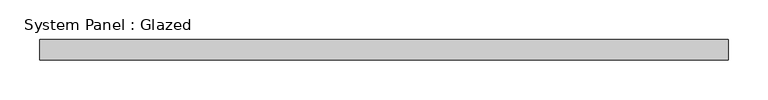
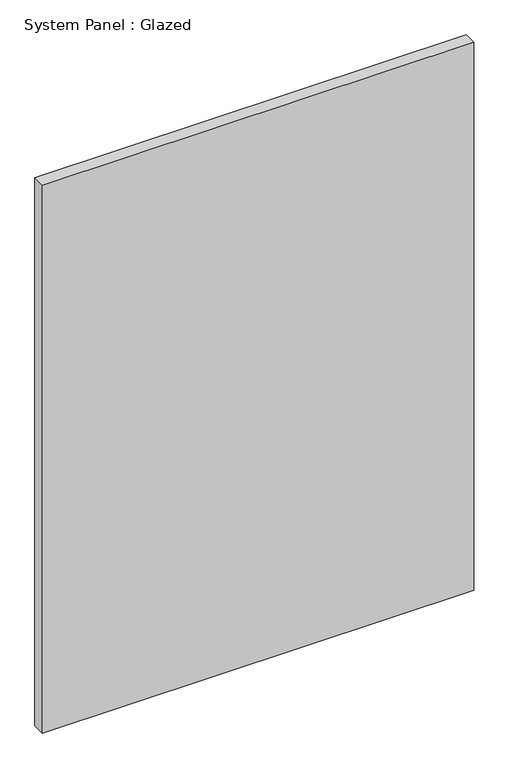
"""IFC4 building model written with IfcOpenShell, lengths in millimetres: plate geometry, System Panel : Glazed."""

from ifc_helpers import new_model, si_unit, origin, origin_with_axes, place, context, project, spatial, polyline, outline, extrude, source, transform, mapped, element, save


def system_panel_glazed_e6c99a0d(model_context):
    return source(origin(), model_context, "Body", "SweptSolid", [
        extrude(outline(polyline([(430.2331274, 19.05), (-430.2331274, 19.05), (-430.2331274, 44.45), (430.2331274, 44.45), (430.2331274, 19.05)])), origin_with_axes(), (0.0, 0.0, 1.0), 1155.7),
    ])


if __name__ == "__main__":
    model = new_model("IFC4")
    model_context = context("Model", 3, world=origin())
    ifc_project = project(units=[si_unit("LENGTHUNIT", "METRE", prefix="MILLI")], contexts=[model_context])
    site = spatial("IfcSite", under=ifc_project)
    building = spatial("IfcBuilding", under=site)
    placement = place(None, origin())
    system_panel_glazed_shape = system_panel_glazed_e6c99a0d(model_context)
    element("IfcPlate", 1, ObjectType="System Panel : Glazed", at=placement, inside=building, context=model_context, shape_type="MappedRepresentation", body=[
        mapped(system_panel_glazed_shape, transform((0.0, 0.0, 0.0), x_axis=(1.0, 0.0, 0.0), y_axis=(0.0, 1.0, 0.0), z_axis=(0.0, 0.0, 1.0))),
    ])
    save(model, "model.ifc")

# Revit data of these elements
# Type "System Panel : Glazed"
#   Construction Type Id = "GSP4R"
#   Analytic Construction = "1/8 in Pilkington single glazing"
#   Visual Light Transmittance = 0.9
#   Solar Heat Gain Coefficient = 0.86
#   Heat Transfer Coefficient (U) = 1.18115 BTU/(h·ft²·°F)
# Element 1 (IfcPlate, "System Panel : Glazed")
#   Materials on its faces: "Glass"
# Materials
#   "Glass": class "Glass", colour RGB 0 128 192, transparency 0.75, Description = "Soda Lime Glass", Cost = 0
